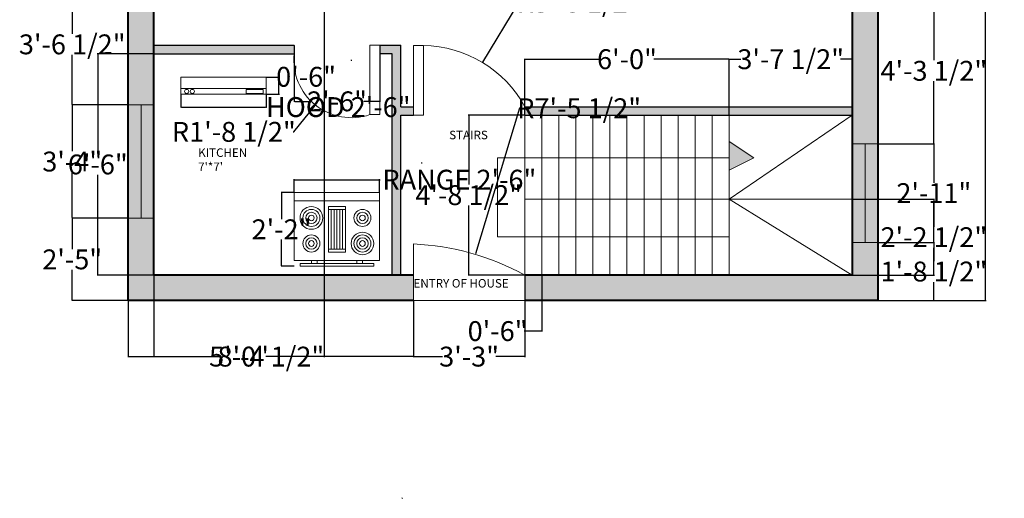
# Model space of a CAD drawing. Units: inches. Extents: x 4466 to 4826, y 3691 to 4152.
# Tile 1 of 4: x 4479 to 4826, y 3691 to 3859. Entities that reach past the tile are written whole.
import ezdxf

# ---------------------------------------------------------------- set-up
doc = ezdxf.new("R2010")
doc.units = ezdxf.units.IN
doc.header["$MEASUREMENT"] = 0
for name, color, linetype, lineweight in [('A-ANNO-DIMS', 2, 'Continuous', 13), ('A-ANNO-TEXT', 7, 'Continuous', 18), ('A-DOOR', 3, 'Continuous', 18), ('A-FLOR-FIXT', 8, 'Continuous', 18), ('A-GLAZ', 4, 'Continuous', 13), ('A-GLAZ-PATT', 9, 'Continuous', 13), ('A-STAI', 7, 'Continuous', 18), ('A-STAI-PATT', 116, 'Continuous', 13), ('A-TEXT-ROOM', 7, 'Continuous', 18), ('A-WALL-EXTR', 7, 'Continuous', 40), ('A-WALL-INTR', 7, 'Continuous', 25), ('A-WALL-PATT', 251, 'Continuous', 13)]:
    doc.layers.add(name, color=color, linetype=linetype, lineweight=lineweight)
doc.styles.get("Standard").update_dxf_attribs({"font": 'arial.ttf'})
doc.dimstyles.get("Standard").update_dxf_attribs({"dimtxt": 7, "dimasz": 0.18, "dimexe": 0.18, "dimexo": 0.0625, "dimgap": 0.09, "dimtad": 0, "dimtih": 1, "dimtoh": 1, "dimdec": 0, "dimzin": 0, "dimdsep": 46, "dimlunit": 3, "dimtxsty": 'Standard', "dimcen": 0.09, "dimadec": 0, "dimazin": 0, "dimtfac": 1, "dimtdec": 0, "dimtofl": 0, "dimtmove": 0, "dimatfit": 3, "dimfxl": 1, "dimtolj": 1, "dimtzin": 0, "dimarcsym": 0})

# ---------------------------------------------------------------- blocks, each defined once
blk = doc.blocks.new('Range-Oven - 30 in top')
for p, q in [((0, -3), (30, -3)), ((12, -6), (18, -6)), ((13, -20), (13, -6)), ((14, -6), (14, -20)), ((15, -20), (15, -6)), ((16, -6), (16, -20)), ((17, -20), (17, -6)), ((18, -20), (12, -20)), ((6, -24), (6, -25)), ((8, -25), (8, -24)), ((22, -25), (22, -24)), ((24, -24), (24, -25))]:
    blk.add_line(p, q)
for points in [[(0, -24), (0, 0), (30, 0), (30, -24)], [(12, -21), (12, -5), (18, -5), (18, -21)], [(2, -26), (2, -25), (28, -25), (28, -26)]]:
    blk.add_lwpolyline(points, close=True)
for centre, radius in [((6, -9), 4), ((6, -9), 3), ((24, -9), 3), ((6, -9), 2), ((6, -9), 1), ((24, -9), 2), ((24, -9), 1), ((6, -18), 3), ((6, -18), 2), ((6, -18), 1), ((24, -18), 4), ((24, -18), 3), ((24, -18), 2), ((24, -18), 1)]:
    blk.add_circle(centre, radius)
blk = doc.blocks.new('Range Hood - 30 in front')
blk.add_line((0, -4), (30.0001, -4))
for points in [[(0, -6), (0, 0), (30.0001, 0), (30.0001, -6)], [(23, -5.75), (23, -4.25), (29, -4.25), (29, -5.75)]]:
    blk.add_lwpolyline(points, close=True)
for centre in [(2, -5), (4, -5)]:
    blk.add_circle(centre, 0.75)
blk = doc.blocks.new('*D6')
at = {"layer": 'A-ANNO-DIMS', "color": 0, "lineweight": -2, "transparency": 16777216}
for p, q in [((4781.8, 4120.28), (4819.85, 4120.28)), ((4819.67, 4120.1), (4819.67, 3943.95)), ((4819.67, 3760.46), (4819.67, 3936.61)), ((4781.8, 3760.28), (4819.85, 3760.28))]:
    blk.add_line(p, q, dxfattribs=at)
at = {"layer": 'A-ANNO-DIMS', "color": 0, "transparency": 16777216}
for points in [[(4819.64, 4120.1), (4819.7, 4120.1), (4819.67, 4120.28)], [(4819.64, 3760.46), (4819.7, 3760.46), (4819.67, 3760.28)]]:
    blk.add_solid(points, dxfattribs=at)
at = {"layer": 'Defpoints', "color": 0, "transparency": 16777216}
for p in [(4781.73, 4120.28), (4781.73, 3760.28), (4819.67, 3760.28)]:
    blk.add_point(p, dxfattribs=at)
at = {"layer": 'A-ANNO-DIMS', "color": 0, "transparency": 16777216, "insert": (4819.67, 3940.28), "char_height": 7, "attachment_point": 5}
blk.add_mtext("\\A1;30'", dxfattribs=at)
blk = doc.blocks.new('*D14')
at = {"layer": 'A-ANNO-DIMS', "color": 0, "lineweight": -2, "transparency": 16777216}
for p, q in [((4576.21, 3798.47), (4576.21, 3803.09)), ((4576.39, 3802.91), (4606.03, 3802.91)), ((4606.21, 3798.47), (4606.21, 3803.09)), ((4606.21, 3802.91), (4606.39, 3802.91))]:
    blk.add_line(p, q, dxfattribs=at)
at = {"layer": 'A-ANNO-DIMS', "color": 0, "transparency": 16777216}
for points in [[(4576.39, 3802.94), (4576.39, 3802.88), (4576.21, 3802.91)], [(4606.03, 3802.94), (4606.03, 3802.88), (4606.21, 3802.91)]]:
    blk.add_solid(points, dxfattribs=at)
at = {"layer": 'Defpoints', "color": 0, "transparency": 16777216}
for p in [(4606.21, 3802.91), (4576.21, 3798.41), (4606.21, 3798.41)]:
    blk.add_point(p, dxfattribs=at)
at = {"layer": 'A-ANNO-DIMS', "color": 0, "transparency": 16777216, "insert": (4634.35, 3802.91), "char_height": 7, "attachment_point": 5}
blk.add_mtext('\\A1;RANGE 2\'-6"', dxfattribs=at)
blk = doc.blocks.new('*D15')
at = {"layer": 'A-ANNO-DIMS', "color": 0, "lineweight": -2, "transparency": 16777216}
for p, q in [((4576.15, 3798.41), (4571.53, 3798.41)), ((4571.71, 3798.23), (4571.71, 3789.02)), ((4571.71, 3772.59), (4571.71, 3781.81)), ((4576.15, 3772.41), (4571.53, 3772.41))]:
    blk.add_line(p, q, dxfattribs=at)
at = {"layer": 'A-ANNO-DIMS', "color": 0, "transparency": 16777216}
for points in [[(4571.68, 3798.23), (4571.74, 3798.23), (4571.71, 3798.41)], [(4571.68, 3772.59), (4571.74, 3772.59), (4571.71, 3772.41)]]:
    blk.add_solid(points, dxfattribs=at)
at = {"layer": 'Defpoints', "color": 0, "transparency": 16777216}
for p in [(4571.71, 3798.41), (4576.21, 3798.41), (4576.21, 3772.41)]:
    blk.add_point(p, dxfattribs=at)
at = {"layer": 'A-ANNO-DIMS', "color": 0, "transparency": 16777216, "insert": (4571.71, 3785.41), "char_height": 7, "attachment_point": 5}
blk.add_mtext('\\A1;2\'-2"', dxfattribs=at)
blk = doc.blocks.new('*D16')
at = {"layer": 'A-ANNO-DIMS', "color": 0, "lineweight": -2, "transparency": 16777216}
for p, q in [((4536.28, 3832.95), (4536.28, 3828.33)), ((4566.28, 3832.95), (4566.28, 3828.33)), ((4536.46, 3828.51), (4566.1, 3828.51)), ((4566.28, 3828.51), (4566.46, 3828.51))]:
    blk.add_line(p, q, dxfattribs=at)
at = {"layer": 'A-ANNO-DIMS', "color": 0, "transparency": 16777216}
for points in [[(4536.46, 3828.54), (4536.46, 3828.48), (4536.28, 3828.51)], [(4566.1, 3828.54), (4566.1, 3828.48), (4566.28, 3828.51)]]:
    blk.add_solid(points, dxfattribs=at)
at = {"layer": 'Defpoints', "color": 0, "transparency": 16777216}
for p in [(4536.28, 3833.01), (4566.28, 3833.01), (4566.28, 3828.51)]:
    blk.add_point(p, dxfattribs=at)
at = {"layer": 'A-ANNO-DIMS', "color": 0, "transparency": 16777216, "insert": (4591.69, 3828.51), "char_height": 7, "attachment_point": 5}
blk.add_mtext('\\A1;HOOD 2\'-6"', dxfattribs=at)
blk = doc.blocks.new('*D17')
at = {"layer": 'A-ANNO-DIMS', "color": 0, "lineweight": -2, "transparency": 16777216}
for p, q in [((4566.34, 3839.01), (4570.96, 3839.01)), ((4570.78, 3839.01), (4570.78, 3839.19)), ((4570.78, 3839.19), (4570.96, 3839.19)), ((4570.78, 3833.19), (4570.78, 3838.83)), ((4566.34, 3833.01), (4570.96, 3833.01))]:
    blk.add_line(p, q, dxfattribs=at)
at = {"layer": 'A-ANNO-DIMS', "color": 0, "transparency": 16777216}
for points in [[(4570.75, 3838.83), (4570.81, 3838.83), (4570.78, 3839.01)], [(4570.75, 3833.19), (4570.81, 3833.19), (4570.78, 3833.01)]]:
    blk.add_solid(points, dxfattribs=at)
at = {"layer": 'Defpoints', "color": 0, "transparency": 16777216}
for p in [(4566.28, 3839.01), (4570.78, 3839.01), (4566.28, 3833.01)]:
    blk.add_point(p, dxfattribs=at)
at = {"layer": 'A-ANNO-DIMS', "color": 0, "transparency": 16777216, "insert": (4580.35, 3839.19), "char_height": 7, "attachment_point": 5}
blk.add_mtext('\\A1;0\'-6"', dxfattribs=at)
blk = doc.blocks.new('*D18')
at = {"layer": 'A-ANNO-DIMS', "color": 0, "lineweight": -2, "transparency": 16777216}
for p, q in [((4517.73, 3760.22), (4517.73, 3740.35)), ((4618.18, 3760.22), (4618.18, 3740.35)), ((4517.91, 3740.53), (4550.4, 3740.53)), ((4618, 3740.53), (4585.51, 3740.53))]:
    blk.add_line(p, q, dxfattribs=at)
at = {"layer": 'A-ANNO-DIMS', "color": 0, "transparency": 16777216}
for points in [[(4517.91, 3740.56), (4517.91, 3740.5), (4517.73, 3740.53)], [(4618, 3740.56), (4618, 3740.5), (4618.18, 3740.53)]]:
    blk.add_solid(points, dxfattribs=at)
at = {"layer": 'Defpoints', "color": 0, "transparency": 16777216}
for p in [(4517.73, 3760.28), (4618.18, 3760.28), (4618.18, 3740.53)]:
    blk.add_point(p, dxfattribs=at)
at = {"layer": 'A-ANNO-DIMS', "color": 0, "transparency": 16777216, "insert": (4567.96, 3740.53), "char_height": 7, "attachment_point": 5}
blk.add_mtext('\\A1;8\'-4 1/2"', dxfattribs=at)
blk = doc.blocks.new('*D19')
at = {"layer": 'A-ANNO-DIMS', "color": 0, "lineweight": -2, "transparency": 16777216}
for p, q in [((4618.18, 3760.22), (4618.18, 3740.35)), ((4657.39, 3760.22), (4657.39, 3740.35)), ((4618.36, 3740.53), (4628.39, 3740.53)), ((4657.21, 3740.53), (4647.18, 3740.53))]:
    blk.add_line(p, q, dxfattribs=at)
at = {"layer": 'A-ANNO-DIMS', "color": 0, "transparency": 16777216}
for points in [[(4618.36, 3740.56), (4618.36, 3740.5), (4618.18, 3740.53)], [(4657.21, 3740.56), (4657.21, 3740.5), (4657.39, 3740.53)]]:
    blk.add_solid(points, dxfattribs=at)
at = {"layer": 'Defpoints', "color": 0, "transparency": 16777216}
for p in [(4618.18, 3760.28), (4657.39, 3760.28), (4657.39, 3740.53)]:
    blk.add_point(p, dxfattribs=at)
at = {"layer": 'A-ANNO-DIMS', "color": 0, "transparency": 16777216, "insert": (4637.78, 3740.53), "char_height": 7, "attachment_point": 5}
blk.add_mtext('\\A1;3\'-3"', dxfattribs=at)
blk = doc.blocks.new('*D20')
at = {"layer": 'A-ANNO-DIMS', "color": 0, "lineweight": -2, "transparency": 16777216}
for p, q in [((4517.67, 3789.34), (4497.8, 3789.34)), ((4497.98, 3789.16), (4497.98, 3778.47)), ((4497.98, 3760.46), (4497.98, 3771.14)), ((4517.67, 3760.28), (4497.8, 3760.28))]:
    blk.add_line(p, q, dxfattribs=at)
at = {"layer": 'A-ANNO-DIMS', "color": 0, "transparency": 16777216}
for points in [[(4497.95, 3789.16), (4498.01, 3789.16), (4497.98, 3789.34)], [(4497.95, 3760.46), (4498.01, 3760.46), (4497.98, 3760.28)]]:
    blk.add_solid(points, dxfattribs=at)
at = {"layer": 'Defpoints', "color": 0, "transparency": 16777216}
for p in [(4497.98, 3789.34), (4517.73, 3789.34), (4517.73, 3760.28)]:
    blk.add_point(p, dxfattribs=at)
at = {"layer": 'A-ANNO-DIMS', "color": 0, "transparency": 16777216, "insert": (4497.98, 3774.81), "char_height": 7, "attachment_point": 5}
blk.add_mtext('\\A1;2\'-5"', dxfattribs=at)
blk = doc.blocks.new('*D21')
at = {"layer": 'A-ANNO-DIMS', "color": 0, "lineweight": -2, "transparency": 16777216}
for p, q in [((4517.67, 3829.25), (4497.8, 3829.25)), ((4497.98, 3829.07), (4497.98, 3812.96)), ((4497.98, 3789.52), (4497.98, 3805.63)), ((4517.67, 3789.34), (4497.8, 3789.34))]:
    blk.add_line(p, q, dxfattribs=at)
at = {"layer": 'A-ANNO-DIMS', "color": 0, "transparency": 16777216}
for points in [[(4497.95, 3829.07), (4498.01, 3829.07), (4497.98, 3829.25)], [(4497.95, 3789.52), (4498.01, 3789.52), (4497.98, 3789.34)]]:
    blk.add_solid(points, dxfattribs=at)
at = {"layer": 'Defpoints', "color": 0, "transparency": 16777216}
for p in [(4497.98, 3829.25), (4517.73, 3829.25), (4517.73, 3789.34)]:
    blk.add_point(p, dxfattribs=at)
at = {"layer": 'A-ANNO-DIMS', "color": 0, "transparency": 16777216, "insert": (4497.98, 3809.3), "char_height": 7, "attachment_point": 5}
blk.add_mtext('\\A1;3\'-4"', dxfattribs=at)
blk = doc.blocks.new('*D22')
at = {"layer": 'A-ANNO-DIMS', "color": 0, "lineweight": -2, "transparency": 16777216}
for p, q in [((4517.67, 3871.98), (4497.8, 3871.98)), ((4497.98, 3871.8), (4497.98, 3854.33)), ((4497.98, 3829.43), (4497.98, 3846.9)), ((4517.67, 3829.25), (4497.8, 3829.25))]:
    blk.add_line(p, q, dxfattribs=at)
at = {"layer": 'A-ANNO-DIMS', "color": 0, "transparency": 16777216}
for points in [[(4497.95, 3871.8), (4498.01, 3871.8), (4497.98, 3871.98)], [(4497.95, 3829.43), (4498.01, 3829.43), (4497.98, 3829.25)]]:
    blk.add_solid(points, dxfattribs=at)
at = {"layer": 'Defpoints', "color": 0, "transparency": 16777216}
for p in [(4497.98, 3871.98), (4517.73, 3871.98), (4517.73, 3829.25)]:
    blk.add_point(p, dxfattribs=at)
at = {"layer": 'A-ANNO-DIMS', "color": 0, "transparency": 16777216, "insert": (4497.98, 3850.62), "char_height": 7, "attachment_point": 5}
blk.add_mtext('\\A1;3\'-6 1/2"', dxfattribs=at)
blk = doc.blocks.new('*D28')
at = {"layer": 'A-ANNO-DIMS', "color": 0, "lineweight": -2, "transparency": 16777216}
for p, q in [((4781.8, 3780.77), (4801.66, 3780.77)), ((4801.48, 3780.59), (4801.48, 3774.23)), ((4801.48, 3760.46), (4801.48, 3766.82)), ((4781.8, 3760.28), (4801.66, 3760.28))]:
    blk.add_line(p, q, dxfattribs=at)
at = {"layer": 'A-ANNO-DIMS', "color": 0, "transparency": 16777216}
for points in [[(4801.45, 3780.59), (4801.51, 3780.59), (4801.48, 3780.77)], [(4801.45, 3760.46), (4801.51, 3760.46), (4801.48, 3760.28)]]:
    blk.add_solid(points, dxfattribs=at)
at = {"layer": 'Defpoints', "color": 0, "transparency": 16777216}
for p in [(4781.73, 3780.77), (4781.73, 3760.28), (4801.48, 3760.28)]:
    blk.add_point(p, dxfattribs=at)
at = {"layer": 'A-ANNO-DIMS', "color": 0, "transparency": 16777216, "insert": (4801.48, 3770.52), "char_height": 7, "attachment_point": 5}
blk.add_mtext('\\A1;1\'-8 1/2"', dxfattribs=at)
blk = doc.blocks.new('*D29')
at = {"layer": 'A-ANNO-DIMS', "color": 0, "lineweight": -2, "transparency": 16777216}
for p, q in [((4781.8, 3815.6), (4801.66, 3815.6)), ((4801.48, 3815.42), (4801.48, 3801.79)), ((4801.48, 3780.95), (4801.48, 3794.58)), ((4781.8, 3780.77), (4801.66, 3780.77))]:
    blk.add_line(p, q, dxfattribs=at)
at = {"layer": 'A-ANNO-DIMS', "color": 0, "transparency": 16777216}
for points in [[(4801.45, 3815.42), (4801.51, 3815.42), (4801.48, 3815.6)], [(4801.45, 3780.95), (4801.51, 3780.95), (4801.48, 3780.77)]]:
    blk.add_solid(points, dxfattribs=at)
at = {"layer": 'Defpoints', "color": 0, "transparency": 16777216}
for p in [(4781.73, 3815.6), (4781.73, 3780.77), (4801.48, 3780.77)]:
    blk.add_point(p, dxfattribs=at)
at = {"layer": 'A-ANNO-DIMS', "color": 0, "transparency": 16777216, "insert": (4801.48, 3798.18), "char_height": 7, "attachment_point": 5}
blk.add_mtext('\\A1;2\'-11"', dxfattribs=at)
blk = doc.blocks.new('*D30')
at = {"layer": 'A-ANNO-DIMS', "color": 0, "lineweight": -2, "transparency": 16777216}
for p, q in [((4781.8, 3867), (4801.66, 3867)), ((4801.48, 3866.82), (4801.48, 3845.01)), ((4801.48, 3815.78), (4801.48, 3837.59)), ((4781.8, 3815.6), (4801.66, 3815.6))]:
    blk.add_line(p, q, dxfattribs=at)
at = {"layer": 'A-ANNO-DIMS', "color": 0, "transparency": 16777216}
for points in [[(4801.45, 3866.82), (4801.51, 3866.82), (4801.48, 3867)], [(4801.45, 3815.78), (4801.51, 3815.78), (4801.48, 3815.6)]]:
    blk.add_solid(points, dxfattribs=at)
at = {"layer": 'Defpoints', "color": 0, "transparency": 16777216}
for p in [(4781.73, 3867), (4781.73, 3815.6), (4801.48, 3815.6)]:
    blk.add_point(p, dxfattribs=at)
at = {"layer": 'A-ANNO-DIMS', "color": 0, "transparency": 16777216, "insert": (4801.48, 3841.3), "char_height": 7, "attachment_point": 5}
blk.add_mtext('\\A1;4\'-3 1/2"', dxfattribs=at)
blk = doc.blocks.new('*D36')
at = {"layer": 'A-ANNO-DIMS', "color": 0, "lineweight": -2, "transparency": 16777216}
for p, q in [((4657.32, 3825.64), (4637.46, 3825.64)), ((4637.64, 3825.46), (4637.64, 3801.17)), ((4637.64, 3769.46), (4637.64, 3793.75)), ((4657.32, 3769.28), (4637.46, 3769.28))]:
    blk.add_line(p, q, dxfattribs=at)
at = {"layer": 'A-ANNO-DIMS', "color": 0, "transparency": 16777216}
for points in [[(4637.61, 3825.46), (4637.67, 3825.46), (4637.64, 3825.64)], [(4637.61, 3769.46), (4637.67, 3769.46), (4637.64, 3769.28)]]:
    blk.add_solid(points, dxfattribs=at)
at = {"layer": 'Defpoints', "color": 0, "transparency": 16777216}
for p in [(4637.64, 3825.64), (4657.39, 3825.64), (4657.39, 3769.28)]:
    blk.add_point(p, dxfattribs=at)
at = {"layer": 'A-ANNO-DIMS', "color": 0, "transparency": 16777216, "insert": (4637.64, 3797.46), "char_height": 7, "attachment_point": 5}
blk.add_mtext('\\A1;4\'-8 1/2"', dxfattribs=at)
blk = doc.blocks.new('*D37')
at = {"layer": 'A-ANNO-DIMS', "color": 0, "lineweight": -2, "transparency": 16777216}
for p, q in [((4657.39, 3825.7), (4657.39, 3845.57)), ((4657.57, 3845.39), (4683.97, 3845.39)), ((4729.21, 3845.39), (4702.8, 3845.39)), ((4729.39, 3825.7), (4729.39, 3845.57))]:
    blk.add_line(p, q, dxfattribs=at)
at = {"layer": 'A-ANNO-DIMS', "color": 0, "transparency": 16777216}
for points in [[(4657.57, 3845.42), (4657.57, 3845.36), (4657.39, 3845.39)], [(4729.21, 3845.42), (4729.21, 3845.36), (4729.39, 3845.39)]]:
    blk.add_solid(points, dxfattribs=at)
at = {"layer": 'Defpoints', "color": 0, "transparency": 16777216}
for p in [(4729.39, 3845.39), (4657.39, 3825.64), (4729.39, 3825.64)]:
    blk.add_point(p, dxfattribs=at)
at = {"layer": 'A-ANNO-DIMS', "color": 0, "transparency": 16777216, "insert": (4693.39, 3845.39), "char_height": 7, "attachment_point": 5}
blk.add_mtext('\\A1;6\'-0"', dxfattribs=at)
blk = doc.blocks.new('*D38')
at = {"layer": 'A-ANNO-DIMS', "color": 0, "lineweight": -2, "transparency": 16777216}
for p, q in [((4729.39, 3825.7), (4729.39, 3845.57)), ((4729.57, 3845.39), (4733.51, 3845.39)), ((4772.55, 3845.39), (4768.61, 3845.39)), ((4772.73, 3825.7), (4772.73, 3845.57))]:
    blk.add_line(p, q, dxfattribs=at)
at = {"layer": 'A-ANNO-DIMS', "color": 0, "transparency": 16777216}
for points in [[(4729.57, 3845.42), (4729.57, 3845.36), (4729.39, 3845.39)], [(4772.55, 3845.42), (4772.55, 3845.36), (4772.73, 3845.39)]]:
    blk.add_solid(points, dxfattribs=at)
at = {"layer": 'Defpoints', "color": 0, "transparency": 16777216}
for p in [(4772.73, 3845.39), (4729.39, 3825.64), (4772.73, 3825.64)]:
    blk.add_point(p, dxfattribs=at)
at = {"layer": 'A-ANNO-DIMS', "color": 0, "transparency": 16777216, "insert": (4751.06, 3845.39), "char_height": 7, "attachment_point": 5}
blk.add_mtext('\\A1;3\'-7 1/2"', dxfattribs=at)
blk = doc.blocks.new('*D39')
at = {"layer": 'A-ANNO-DIMS', "color": 0, "lineweight": -2, "transparency": 16777216}
for p, q in [((4772.8, 3795.99), (4801.66, 3795.99)), ((4801.48, 3795.81), (4801.48, 3786.34)), ((4801.48, 3769.46), (4801.48, 3778.93)), ((4772.8, 3769.28), (4801.66, 3769.28))]:
    blk.add_line(p, q, dxfattribs=at)
at = {"layer": 'A-ANNO-DIMS', "color": 0, "transparency": 16777216}
for points in [[(4801.45, 3795.81), (4801.51, 3795.81), (4801.48, 3795.99)], [(4801.45, 3769.46), (4801.51, 3769.46), (4801.48, 3769.28)]]:
    blk.add_solid(points, dxfattribs=at)
at = {"layer": 'Defpoints', "color": 0, "transparency": 16777216}
for p in [(4772.73, 3795.99), (4801.48, 3795.99), (4772.73, 3769.28)]:
    blk.add_point(p, dxfattribs=at)
at = {"layer": 'A-ANNO-DIMS', "color": 0, "transparency": 16777216, "insert": (4801.48, 3782.63), "char_height": 7, "attachment_point": 5}
blk.add_mtext('\\A1;2\'-2 1/2"', dxfattribs=at)
blk = doc.blocks.new('*D40')
at = {"layer": 'A-ANNO-DIMS', "color": 0, "lineweight": -2, "transparency": 16777216}
for p, q in [((4657.39, 3769.22), (4657.39, 3749.35)), ((4663.39, 3769.22), (4663.39, 3749.35)), ((4657.39, 3749.53), (4657.21, 3749.53)), ((4663.21, 3749.53), (4657.57, 3749.53))]:
    blk.add_line(p, q, dxfattribs=at)
at = {"layer": 'A-ANNO-DIMS', "color": 0, "transparency": 16777216}
for points in [[(4657.57, 3749.56), (4657.57, 3749.5), (4657.39, 3749.53)], [(4663.21, 3749.56), (4663.21, 3749.5), (4663.39, 3749.53)]]:
    blk.add_solid(points, dxfattribs=at)
at = {"layer": 'Defpoints', "color": 0, "transparency": 16777216}
for p in [(4657.39, 3769.28), (4663.39, 3769.28), (4657.39, 3749.53)]:
    blk.add_point(p, dxfattribs=at)
at = {"layer": 'A-ANNO-DIMS', "color": 0, "transparency": 16777216, "insert": (4647.81, 3749.53), "char_height": 7, "attachment_point": 5}
blk.add_mtext('\\A1;0\'-6"', dxfattribs=at)
blk = doc.blocks.new('*D41')
at = {"layer": 'A-ANNO-DIMS', "color": 0, "lineweight": -2, "transparency": 16777216}
for p, q in [((4526.73, 3928.22), (4526.73, 3740.35)), ((4586.73, 3928.22), (4586.73, 3740.35)), ((4526.91, 3740.53), (4547.34, 3740.53)), ((4586.55, 3740.53), (4566.13, 3740.53))]:
    blk.add_line(p, q, dxfattribs=at)
at = {"layer": 'A-ANNO-DIMS', "color": 0, "transparency": 16777216}
for points in [[(4526.91, 3740.56), (4526.91, 3740.5), (4526.73, 3740.53)], [(4586.55, 3740.56), (4586.55, 3740.5), (4586.73, 3740.53)]]:
    blk.add_solid(points, dxfattribs=at)
at = {"layer": 'Defpoints', "color": 0, "transparency": 16777216}
for p in [(4526.73, 3928.28), (4586.73, 3928.28), (4586.73, 3740.53)]:
    blk.add_point(p, dxfattribs=at)
at = {"layer": 'A-ANNO-DIMS', "color": 0, "transparency": 16777216, "insert": (4556.73, 3740.53), "char_height": 7, "attachment_point": 5}
blk.add_mtext('\\A1;5\'-0"', dxfattribs=at)
blk = doc.blocks.new('*D46')
at = {"layer": 'A-ANNO-DIMS', "color": 0, "lineweight": -2, "transparency": 16777216}
for p, q in [((4526.67, 3847.28), (4506.8, 3847.28)), ((4506.98, 3847.1), (4506.98, 3811.94)), ((4506.98, 3769.46), (4506.98, 3804.62)), ((4526.67, 3769.28), (4506.8, 3769.28))]:
    blk.add_line(p, q, dxfattribs=at)
at = {"layer": 'A-ANNO-DIMS', "color": 0, "transparency": 16777216}
for points in [[(4506.95, 3847.1), (4507.01, 3847.1), (4506.98, 3847.28)], [(4506.95, 3769.46), (4507.01, 3769.46), (4506.98, 3769.28)]]:
    blk.add_solid(points, dxfattribs=at)
at = {"layer": 'Defpoints', "color": 0, "transparency": 16777216}
for p in [(4506.98, 3847.28), (4526.73, 3847.28), (4526.73, 3769.28)]:
    blk.add_point(p, dxfattribs=at)
at = {"layer": 'A-ANNO-DIMS', "color": 0, "transparency": 16777216, "insert": (4506.98, 3808.28), "char_height": 7, "attachment_point": 5}
blk.add_mtext('\\A1;6\'-6"', dxfattribs=at)
blk = doc.blocks.new('*D53')
at = {"layer": 'A-ANNO-DIMS', "color": 0, "lineweight": -2, "transparency": 16777216}
for p, q in [((4576.17, 3850.22), (4576.17, 3830.35)), ((4606.34, 3850.22), (4606.34, 3830.35)), ((4576.35, 3830.53), (4581.8, 3830.53)), ((4606.16, 3830.53), (4600.71, 3830.53))]:
    blk.add_line(p, q, dxfattribs=at)
at = {"layer": 'A-ANNO-DIMS', "color": 0, "transparency": 16777216}
for points in [[(4576.35, 3830.56), (4576.35, 3830.5), (4576.17, 3830.53)], [(4606.16, 3830.56), (4606.16, 3830.5), (4606.34, 3830.53)]]:
    blk.add_solid(points, dxfattribs=at)
at = {"layer": 'Defpoints', "color": 0, "transparency": 16777216}
for p in [(4576.17, 3850.28), (4606.34, 3850.28), (4576.17, 3830.53)]:
    blk.add_point(p, dxfattribs=at)
at = {"layer": 'A-ANNO-DIMS', "color": 0, "transparency": 16777216, "insert": (4591.25, 3830.53), "char_height": 7, "attachment_point": 5}
blk.add_mtext('\\A1;2\'-6"', dxfattribs=at)
blk = doc.blocks.new('*D58')
at = {"layer": 'A-ANNO-DIMS', "color": 0, "lineweight": -2, "transparency": 16777216}
for p, q in [((4655.25, 3865.47), (4642.54, 3844.4)), ((4655.43, 3865.47), (4655.25, 3865.47)), ((4621.03, 3808.87), (4621.21, 3808.87)), ((4621.12, 3808.78), (4621.12, 3808.96))]:
    blk.add_line(p, q, dxfattribs=at)
at = {"layer": 'A-ANNO-DIMS', "color": 0, "transparency": 16777216}
blk.add_solid([(4642.52, 3844.41), (4642.57, 3844.38), (4642.45, 3844.24)], dxfattribs=at)
at = {"layer": 'Defpoints', "color": 0, "transparency": 16777216}
for p in [(4642.45, 3844.24), (4621.12, 3808.87)]:
    blk.add_point(p, dxfattribs=at)
at = {"layer": 'A-ANNO-DIMS', "color": 0, "transparency": 16777216, "insert": (4676.33, 3865.47), "char_height": 7, "attachment_point": 5}
blk.add_mtext('\\A1;R3\'-5 1/2"', dxfattribs=at)
blk = doc.blocks.new('*D59')
at = {"layer": 'A-ANNO-DIMS', "color": 0, "lineweight": -2, "transparency": 16777216}
for p, q in [((4596.23, 3845.05), (4596.41, 3845.05)), ((4596.32, 3844.96), (4596.32, 3845.14)), ((4575.99, 3819.77), (4583.5, 3829.11)), ((4575.81, 3819.77), (4575.99, 3819.77))]:
    blk.add_line(p, q, dxfattribs=at)
at = {"layer": 'A-ANNO-DIMS', "color": 0, "transparency": 16777216}
blk.add_solid([(4583.47, 3829.13), (4583.52, 3829.09), (4583.61, 3829.25)], dxfattribs=at)
at = {"layer": 'Defpoints', "color": 0, "transparency": 16777216}
for p in [(4596.32, 3845.05), (4583.61, 3829.25)]:
    blk.add_point(p, dxfattribs=at)
at = {"layer": 'A-ANNO-DIMS', "color": 0, "transparency": 16777216, "insert": (4554.91, 3819.77), "char_height": 7, "attachment_point": 5}
blk.add_mtext('\\A1;R1\'-8 1/2"', dxfattribs=at)
blk = doc.blocks.new('*D64')
at = {"layer": 'A-ANNO-DIMS', "color": 0, "lineweight": -2, "transparency": 16777216}
for p, q in [((4655.47, 3828.09), (4640.07, 3776.73)), ((4655.65, 3828.09), (4655.47, 3828.09)), ((4614.16, 3690.66), (4614.34, 3690.66)), ((4614.25, 3690.57), (4614.25, 3690.75))]:
    blk.add_line(p, q, dxfattribs=at)
at = {"layer": 'A-ANNO-DIMS', "color": 0, "transparency": 16777216}
blk.add_solid([(4640.04, 3776.73), (4640.1, 3776.72), (4640.02, 3776.55)], dxfattribs=at)
at = {"layer": 'Defpoints', "color": 0, "transparency": 16777216}
for p in [(4640.02, 3776.55), (4614.25, 3690.66)]:
    blk.add_point(p, dxfattribs=at)
at = {"layer": 'A-ANNO-DIMS', "color": 0, "transparency": 16777216, "insert": (4676.55, 3828.09), "char_height": 7, "attachment_point": 5}
blk.add_mtext('\\A1;R7\'-5 1/2"', dxfattribs=at)

msp = doc.modelspace()

# ---------------------------------------------------------------- hatches: boundary and pattern name
at = {"layer": 'A-GLAZ-PATT'}
h = msp.add_hatch(color=256, dxfattribs=at)
h.dxf.hatch_style = 1
h.paths.add_polyline_path([(4781.73, 3815.6), (4777.23, 3815.6), (4777.23, 3780.77), (4781.73, 3780.77)])
h.paths.add_polyline_path([(4777.23, 3815.6), (4772.73, 3815.6), (4772.73, 3780.77), (4777.23, 3780.77)])
h.paths.add_polyline_path([(4781.73, 3906.43), (4777.23, 3906.43), (4777.23, 3867), (4781.73, 3867)])
h.paths.add_polyline_path([(4777.23, 3906.43), (4772.73, 3906.43), (4772.73, 3867), (4777.23, 3867)])
h.paths.add_polyline_path([(4777.23, 3975.56), (4772.73, 3975.56), (4772.73, 3940.28), (4777.23, 3940.28)])
h.paths.add_polyline_path([(4781.73, 3975.56), (4777.23, 3975.56), (4777.23, 3940.28), (4781.73, 3940.28)])
h.paths.add_polyline_path([(4781.73, 4086.44), (4777.23, 4086.44), (4777.23, 4025.83), (4781.73, 4025.83)])
h.paths.add_polyline_path([(4777.23, 4086.44), (4772.73, 4086.44), (4772.73, 4025.83), (4777.23, 4025.83)])
h.paths.add_polyline_path([(4526.73, 4085.19), (4522.23, 4085.19), (4522.23, 4027.88), (4526.73, 4027.88)])
h.paths.add_polyline_path([(4522.23, 4085.19), (4517.73, 4085.19), (4517.73, 4027.88), (4522.23, 4027.88)])
h.paths.add_polyline_path([(4526.73, 3973.15), (4522.23, 3973.15), (4522.23, 3949.75), (4526.73, 3949.75)])
h.paths.add_polyline_path([(4522.23, 3973.15), (4517.73, 3973.15), (4517.73, 3949.75), (4522.23, 3949.75)])
h.paths.add_polyline_path([(4522.23, 3906.82), (4517.73, 3906.82), (4517.73, 3871.98), (4522.23, 3871.98)])
h.paths.add_polyline_path([(4526.73, 3906.82), (4522.23, 3906.82), (4522.23, 3871.98), (4526.73, 3871.98)])
h.paths.add_polyline_path([(4526.73, 3829.25), (4522.23, 3829.25), (4522.23, 3789.34), (4526.73, 3789.34)])
h.paths.add_polyline_path([(4522.23, 3829.25), (4517.73, 3829.25), (4517.73, 3789.34), (4522.23, 3789.34)])
at = {"layer": 'A-STAI-PATT'}
h = msp.add_hatch(color=256, dxfattribs=at)
h.dxf.hatch_style = 1
h.paths.add_polyline_path([(4738.02, 3810.66), (4729.39, 3816.36), (4729.39, 3806.26)])
at = {"layer": 'A-WALL-PATT'}
h = msp.add_hatch(color=256, dxfattribs=at)
h.dxf.hatch_style = 1
h.paths.add_polyline_path([(4781.73, 4120.28), (4517.73, 4120.28), (4517.73, 4085.19), (4526.73, 4085.19), (4526.73, 4111.28), (4772.73, 4111.28), (4772.73, 4086.44), (4781.73, 4086.44)])
h.paths.add_polyline_path([(4526.73, 4027.88), (4517.73, 4027.88), (4517.73, 3973.15), (4526.73, 3973.15)])
h.paths.add_polyline_path([(4781.73, 4025.83), (4772.73, 4025.83), (4772.73, 3975.56), (4781.73, 3975.56)])
h.paths.add_polyline_path([(4651.73, 4111.28), (4647.73, 4111.28), (4647.73, 3991.28), (4638.9, 3991.28), (4638.9, 3988.28), (4662.75, 3988.28), (4662.75, 3991.28), (4651.73, 3991.28)])
h.paths.add_polyline_path([(4781.73, 3780.77), (4772.73, 3780.77), (4772.73, 3769.28), (4657.39, 3769.28), (4657.39, 3760.28), (4781.73, 3760.28)])
h.paths.add_polyline_path([(4781.73, 3867), (4772.73, 3867), (4772.73, 3815.6), (4781.73, 3815.6)])
h.paths.add_polyline_path([(4781.73, 3940.28), (4772.73, 3940.28), (4772.73, 3906.43), (4781.73, 3906.43)])
h.paths.add_polyline_path([(4526.73, 3949.75), (4517.73, 3949.75), (4517.73, 3906.82), (4526.73, 3906.82)])
h.paths.add_polyline_path([(4526.73, 3871.98), (4517.73, 3871.98), (4517.73, 3829.25), (4526.73, 3829.25)])
h.paths.add_polyline_path([(4618.18, 3769.28), (4526.73, 3769.28), (4526.73, 3789.34), (4517.73, 3789.34), (4517.73, 3760.28), (4618.18, 3760.28)])
h.paths.add_polyline_path([(4576.17, 3850.28), (4526.73, 3850.28), (4526.73, 3847.28), (4576.17, 3847.28)])
h.paths.add_polyline_path([(4613.73, 3825.64), (4618.18, 3825.64), (4618.18, 3828.64), (4613.73, 3828.64), (4613.73, 3850.28), (4610.73, 3850.28), (4606.34, 3850.28), (4606.34, 3847.28), (4610.73, 3847.28), (4610.73, 3769.28), (4613.73, 3769.28)])
h.paths.add_polyline_path([(4772.73, 3828.64), (4657.39, 3828.64), (4657.39, 3825.64), (4772.73, 3825.64)])
h.paths.add_polyline_path([(4589.73, 3988.28), (4586.73, 3988.28), (4586.73, 3928.28), (4589.73, 3928.28)])
h.paths.add_polyline_path([(4712.73, 3956.78), (4709.73, 3956.78), (4709.73, 3925.28), (4772.73, 3925.28), (4772.73, 3928.28), (4712.73, 3928.28)])
h.paths.add_polyline_path([(4772.73, 3991.28), (4705.82, 3991.28), (4705.82, 3988.28), (4772.73, 3988.28)])
h.paths.add_polyline_path([(4559.49, 3991.28), (4526.73, 3991.28), (4526.73, 3988.28), (4559.49, 3988.28)])

# ---------------------------------------------------------------- linework, layer by layer
at = {"layer": 'A-DOOR'}
for p, q in [((4576.17, 3850.28), (4576.17, 3847.28)), ((4606.34, 3850.28), (4602.82, 3850.28)), ((4602.82, 3850.28), (4602.82, 3825.84)), ((4606.34, 3847.28), (4606.34, 3850.28)), ((4621.68, 3850.17), (4618.18, 3850.17)), ((4618.18, 3850.17), (4618.18, 3828.64)), ((4621.68, 3825.64), (4621.68, 3850.17)), ((4606.34, 3847.28), (4606.34, 3825.84)), ((4606.34, 3825.84), (4602.82, 3825.84)), ((4618.18, 3828.64), (4618.18, 3825.64)), ((4618.18, 3825.64), (4621.68, 3825.64)), ((4657.39, 3828.64), (4657.39, 3825.64)), ((4618.18, 3769.28), (4618.18, 3780.25)), ((4618.18, 3769.28), (4618.18, 3760.28)), ((4657.39, 3769.28), (4657.39, 3760.28)), ((4618.18, 3760.28), (4657.39, 3760.28))]:
    msp.add_line(p, q, dxfattribs=at)
for centre, radius, start, end in [((4621.12, 3808.87), 41.31, 28.5976, 89.2197), ((4596.32, 3845.05), 20.28, 173.6771, 288.696), ((4614.25, 3690.66), 89.68, 61.2495, 87.4877)]:
    msp.add_arc(centre, radius, start, end, dxfattribs=at)
at = {"layer": 'A-GLAZ'}
for p, q in [((4517.73, 3829.25), (4526.73, 3829.25)), ((4522.23, 3829.25), (4522.23, 3789.34)), ((4772.73, 3815.6), (4781.73, 3815.6)), ((4777.23, 3815.6), (4777.23, 3780.77)), ((4517.73, 3789.34), (4526.73, 3789.34)), ((4772.73, 3780.77), (4781.73, 3780.77))]:
    msp.add_line(p, q, dxfattribs=at)
at = {"layer": 'A-STAI'}
for p, q in [((4657.39, 3769.28), (4657.39, 3825.64)), ((4663.39, 3769.28), (4663.39, 3825.64)), ((4669.39, 3769.28), (4669.39, 3825.64)), ((4669.39, 3769.28), (4669.39, 3825.64)), ((4675.39, 3769.28), (4675.39, 3825.64)), ((4681.39, 3769.28), (4681.39, 3825.64)), ((4687.39, 3769.28), (4687.39, 3825.64)), ((4693.39, 3769.28), (4693.39, 3825.64)), ((4699.39, 3769.28), (4699.39, 3825.64)), ((4705.39, 3769.28), (4705.39, 3825.64)), ((4711.39, 3769.28), (4711.39, 3825.64)), ((4717.39, 3769.28), (4717.39, 3825.64)), ((4723.39, 3769.28), (4723.39, 3825.64)), ((4729.39, 3769.28), (4729.39, 3825.64)), ((4729.39, 3795.99), (4772.73, 3825.64)), ((4738.02, 3810.66), (4729.39, 3816.36)), ((4647.72, 3782.72), (4647.72, 3810.66)), ((4647.72, 3810.66), (4729.39, 3810.66)), ((4729.39, 3806.26), (4738.02, 3810.66)), ((4772.73, 3795.99), (4657.39, 3795.99)), ((4772.73, 3769.28), (4729.39, 3795.99)), ((4729.39, 3782.72), (4647.72, 3782.72)), ((4729.39, 3782.72), (4729.39, 3782.72))]:
    msp.add_line(p, q, dxfattribs=at)
at = {"layer": 'A-WALL-EXTR'}
for p, q in [((4526.73, 3769.28), (4526.73, 4111.28)), ((4772.73, 4111.28), (4772.73, 3769.28)), ((4618.18, 3769.28), (4526.73, 3769.28)), ((4772.73, 3769.28), (4657.39, 3769.28))]:
    msp.add_line(p, q, dxfattribs=at)
msp.add_lwpolyline([(4618.18, 3760.28), (4517.73, 3760.28), (4517.73, 4120.28), (4781.73, 4120.28), (4781.73, 3760.28), (4657.39, 3760.28)], dxfattribs=at)
at = {"layer": 'A-WALL-INTR'}
for p, q in [((4526.73, 3850.28), (4576.17, 3850.28)), ((4606.34, 3850.28), (4610.73, 3850.28)), ((4610.73, 3850.28), (4613.73, 3850.28)), ((4613.73, 3828.64), (4613.73, 3850.28)), ((4526.73, 3847.28), (4576.17, 3847.28)), ((4610.73, 3847.28), (4606.34, 3847.28)), ((4610.73, 3769.28), (4610.73, 3847.28)), ((4613.73, 3828.64), (4618.18, 3828.64)), ((4613.73, 3769.28), (4613.73, 3825.64)), ((4613.73, 3825.64), (4618.18, 3825.64)), ((4657.39, 3828.64), (4772.73, 3828.64)), ((4657.39, 3825.64), (4772.73, 3825.64))]:
    msp.add_line(p, q, dxfattribs=at)

# ---------------------------------------------------------------- block references
at = {"layer": 'A-FLOR-FIXT'}
for name, p in [('Range Hood - 30 in front', (4536.28, 3839.01)), ('Range-Oven - 30 in top', (4576.21, 3798.41))]:
    msp.add_blockref(name, p, dxfattribs=at)

# ---------------------------------------------------------------- texts
at = {"layer": 'A-ANNO-TEXT', "insert": (4618.18, 3767.88), "char_height": 3, "attachment_point": 1}
msp.add_mtext_dynamic_manual_height_columns('ENTRY OF HOUSE', width=77.4792, gutter_width=1, heights=[0], dxfattribs=at)
at = {"layer": 'A-STAI', "insert": (4630.76, 3820.17), "char_height": 3, "attachment_point": 1}
msp.add_mtext_dynamic_manual_height_columns('STAIRS', width=77.4792, gutter_width=1, heights=[0], dxfattribs=at)
at = {"layer": 'A-TEXT-ROOM', "insert": (4542.35, 3813.95), "char_height": 3, "attachment_point": 1}
msp.add_mtext_dynamic_manual_height_columns("KITCHEN\\P7'*7'", width=77.4792, gutter_width=1, heights=[0], dxfattribs=at)

# ---------------------------------------------------------------- dimensions: what is measured, and where the dimension line sits
at = {"layer": 'A-ANNO-DIMS'}
for base, p1, p2, angle, override, picture, middle in [((4819.67, 3760.28), (4781.73, 4120.28), (4781.73, 3760.28), 90, {"dimclrd": 0, "dimclre": 0, "dimclrt": 0}, '*D6', (4819.67, 3940.28)), ((4497.98, 3871.98), (4517.73, 3829.25), (4517.73, 3871.98), 90, {"dimdec": 1, "dimlfac": 1, "dimrnd": 0, "dimzin": 1, "dimdsep": 46, "dimlunit": 4, "dimfrac": 2}, '*D22', (4497.98, 3850.62)), ((4801.48, 3815.6), (4781.73, 3867), (4781.73, 3815.6), 270, {"dimdec": 1, "dimlfac": 1, "dimrnd": 0, "dimzin": 1, "dimdsep": 46, "dimlunit": 4, "dimfrac": 2}, '*D30', (4801.48, 3841.3)), ((4772.73, 3845.39), (4729.39, 3825.64), (4772.73, 3825.64), 0, {"dimdec": 1, "dimlfac": 1, "dimrnd": 0, "dimzin": 1, "dimdsep": 46, "dimlunit": 4, "dimfrac": 2}, '*D38', (4751.06, 3845.39)), ((4576.17, 3830.53), (4606.34, 3850.28), (4576.17, 3850.28), 180, {"dimdec": 1, "dimlfac": 1, "dimrnd": 0, "dimzin": 1, "dimdsep": 46, "dimlunit": 4, "dimfrac": 2}, '*D53', (4591.25, 3830.53)), ((4506.98, 3847.28), (4526.73, 3769.28), (4526.73, 3847.28), 90, {"dimdec": 1, "dimlfac": 1, "dimrnd": 0, "dimzin": 1, "dimdsep": 46, "dimlunit": 4, "dimfrac": 2}, '*D46', (4506.98, 3808.28)), ((4570.78, 3839.01), (4566.28, 3833.01), (4566.28, 3839.01), 90, {"dimdec": 1, "dimlfac": 1, "dimrnd": 0, "dimzin": 1, "dimdsep": 46, "dimlunit": 4, "dimfrac": 2}, '*D17', (4580.35, 3839.19)), ((4497.98, 3829.25), (4517.73, 3789.34), (4517.73, 3829.25), 90, {"dimdec": 1, "dimlfac": 1, "dimrnd": 0, "dimzin": 1, "dimdsep": 46, "dimlunit": 4, "dimfrac": 2}, '*D21', (4497.98, 3809.3)), ((4637.64, 3825.64), (4657.39, 3769.28), (4657.39, 3825.64), 90, {"dimdec": 1, "dimlfac": 1, "dimrnd": 0, "dimzin": 1, "dimdsep": 46, "dimlunit": 4, "dimfrac": 2}, '*D36', (4637.64, 3797.46)), ((4801.48, 3780.77), (4781.73, 3815.6), (4781.73, 3780.77), 270, {"dimdec": 1, "dimlfac": 1, "dimrnd": 0, "dimzin": 1, "dimdsep": 46, "dimlunit": 4, "dimfrac": 2}, '*D29', (4801.48, 3798.18)), ((4571.71, 3798.41), (4576.21, 3772.41), (4576.21, 3798.41), 90, {"dimdec": 1, "dimlfac": 1, "dimrnd": 0, "dimzin": 1, "dimdsep": 46, "dimlunit": 4, "dimfrac": 2}, '*D15', (4571.71, 3785.41)), ((4801.48, 3795.99), (4772.73, 3769.28), (4772.73, 3795.99), 90, {"dimdec": 1, "dimlfac": 1, "dimrnd": 0, "dimzin": 1, "dimdsep": 46, "dimlunit": 4, "dimfrac": 2}, '*D39', (4801.48, 3782.63)), ((4497.98, 3789.34), (4517.73, 3760.28), (4517.73, 3789.34), 90, {"dimdec": 1, "dimlfac": 1, "dimrnd": 0, "dimzin": 1, "dimdsep": 46, "dimlunit": 4, "dimfrac": 2}, '*D20', (4497.98, 3774.81)), ((4801.48, 3760.28), (4781.73, 3780.77), (4781.73, 3760.28), 270, {"dimdec": 1, "dimlfac": 1, "dimrnd": 0, "dimzin": 1, "dimdsep": 46, "dimlunit": 4, "dimfrac": 2}, '*D28', (4801.48, 3770.52)), ((4657.39, 3749.53), (4663.39, 3769.28), (4657.39, 3769.28), 180, {"dimdec": 1, "dimlfac": 1, "dimrnd": 0, "dimzin": 1, "dimdsep": 46, "dimlunit": 4, "dimfrac": 2}, '*D40', (4647.81, 3749.53))]:
    dim = msp.add_linear_dim(base=base, p1=p1, p2=p2, angle=angle, dimstyle='Standard', override=override, dxfattribs=at)
    dim.commit()
    dim.dimension.update_dxf_attribs({"geometry": picture, "text_midpoint": middle})
for base, p1, p2, picture, middle in [((4586.73, 3740.53), (4526.73, 3928.28), (4586.73, 3928.28), '*D41', (4556.73, 3740.53)), ((4729.39, 3845.39), (4657.39, 3825.64), (4729.39, 3825.64), '*D37', (4693.39, 3845.39)), ((4618.1825, 3740.5291), (4517.7337, 3760.2791), (4618.1825, 3760.2791), '*D18', (4567.9581, 3740.5291)), ((4657.39, 3740.53), (4618.18, 3760.28), (4657.39, 3760.28), '*D19', (4637.78, 3740.53))]:
    dim = msp.add_linear_dim(base=base, p1=p1, p2=p2, dimstyle='Standard', override={"dimdec": 1, "dimlfac": 1, "dimrnd": 0, "dimzin": 1, "dimdsep": 46, "dimlunit": 4, "dimfrac": 2}, dxfattribs=at)
    dim.commit()
    dim.dimension.update_dxf_attribs({"geometry": picture, "text_midpoint": middle})
for center, mpoint, picture, middle in [((4621.12, 3808.87), (4642.45, 3844.24), '*D58', (4676.33, 3865.47)), ((4596.32, 3845.05), (4583.61, 3829.25), '*D59', (4554.91, 3819.77)), ((4614.25, 3690.66), (4640.02, 3776.55), '*D64', (4676.55, 3828.09))]:
    dim = msp.add_radius_dim(center=center, mpoint=mpoint, dimstyle='Standard', override={"dimdec": 1, "dimlfac": 1, "dimrnd": 0, "dimzin": 1, "dimdsep": 46, "dimlunit": 4, "dimfrac": 2}, dxfattribs=at)
    dim.commit()
    dim.dimension.update_dxf_attribs({"geometry": picture, "text_midpoint": middle, "dimtype": 164})
for base, p1, p2, text, picture, middle in [((4566.28, 3828.51), (4536.28, 3833.01), (4566.28, 3833.01), 'HOOD <>', '*D16', (4591.69, 3828.51)), ((4606.21, 3802.91), (4576.21, 3798.41), (4606.21, 3798.41), 'RANGE <>', '*D14', (4634.35, 3802.91))]:
    dim = msp.add_linear_dim(base=base, p1=p1, p2=p2, text=text, dimstyle='Standard', override={"dimdec": 1, "dimlfac": 1, "dimrnd": 0, "dimzin": 1, "dimdsep": 46, "dimlunit": 4, "dimfrac": 2}, dxfattribs=at)
    dim.commit()
    dim.dimension.update_dxf_attribs({"geometry": picture, "text_midpoint": middle})

doc.saveas('drawing.dxf')
